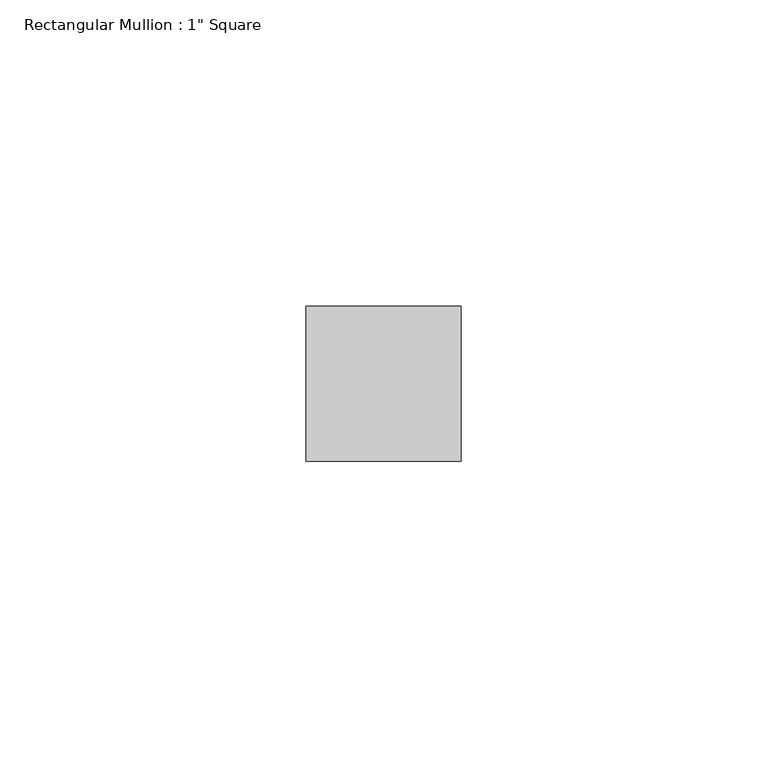
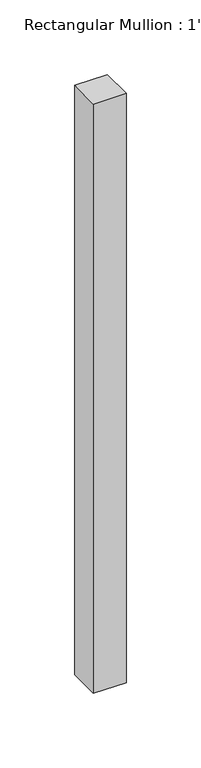
"""IFC4 building model written with IfcOpenShell, lengths in millimetres: member geometry."""

from ifc_helpers import new_model, si_unit, frame, origin, place, context, project, spatial, polyline, outline, extrude, source, transform, mapped, element, save


def member_93b5357b(model_context):
    return source(origin(), model_context, "Body", "SweptSolid", [
        extrude(outline(polyline([(12.7, 12.7), (12.7, -12.7), (-12.7, -12.7), (-12.7, 12.7), (12.7, 12.7)])), frame((0.0, 0.0, -482.6), z_axis=(0.0, 0.0, 1.0), x_axis=(1.0, 0.0, 0.0)), (0.0, 0.0, 1.0), 482.6),
    ])


if __name__ == "__main__":
    model = new_model("IFC4")
    model_context = context("Model", 3, world=origin())
    ifc_project = project(units=[si_unit("LENGTHUNIT", "METRE", prefix="MILLI")], contexts=[model_context])
    site = spatial("IfcSite", under=ifc_project)
    building = spatial("IfcBuilding", under=site)
    placement = place(None, origin())
    member_shape = member_93b5357b(model_context)
    element("IfcMember", 1, ObjectType="Rectangular Mullion : 1\" Square", at=placement, inside=building, context=model_context, shape_type="MappedRepresentation", body=[
        mapped(member_shape, transform((0.0, 0.0, 0.0), x_axis=(1.0, 0.0, 0.0), y_axis=(0.0, 1.0, 0.0), z_axis=(0.0, 0.0, 1.0))),
    ])
    save(model, "model.ifc")

# Revit data of these elements
# Type "Rectangular Mullion : 1\" Square"
#   built-in parameter 1007304 = 0.0833333 (stored number, unit not read)
#   built-in parameter 1007301 = 0.0416667 (stored number, unit not read)
#   built-in parameter 1007300 = 0.0416667 (stored number, unit not read)
# Element 1 (IfcMember, "Rectangular Mullion : 1\" Square")
#   Materials on its faces: "Aluminum"
# Materials
#   "Aluminum": class "Metal", colour RGB 247 247 247, transparency 0, Description = "Aluminum 6061", Cost = 0
